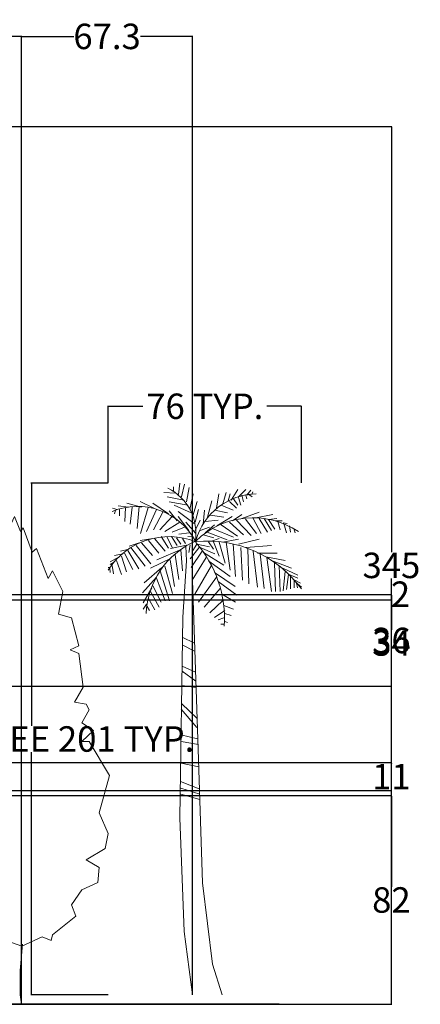
# Model space of a CAD drawing. Units: inches. Extents: x 403 to 1256, y 451 to 842.
# Tile 4 of 4: x 1098 to 1256, y 455 to 842. Entities that reach past the tile are written whole.
import ezdxf

# ---------------------------------------------------------------- set-up
doc = ezdxf.new("R2010")
doc.units = ezdxf.units.IN
doc.header["$MEASUREMENT"] = 0
for name, color, linetype, lineweight in [('A-ANNO-DIMS', 2, 'Continuous', 18), ('A-WALL', 7, 'Continuous', 35), ('PLANTS', 3, 'Continuous', 18)]:
    doc.layers.add(name, color=color, linetype=linetype, lineweight=lineweight)
doc.styles.get("Standard").update_dxf_attribs({"font": 'arial.ttf'})
doc.dimstyles.get("Standard").update_dxf_attribs({"dimtxt": 10, "dimasz": 0.18, "dimexe": 0.18, "dimexo": 0.0625, "dimgap": 0.09, "dimtad": 0, "dimtih": 1, "dimtoh": 1, "dimdec": 0, "dimzin": 0, "dimdsep": 46, "dimlunit": 3, "dimtxsty": 'Standard', "dimcen": 0.09, "dimadec": 0, "dimazin": 0, "dimtfac": 1, "dimtdec": 0, "dimtofl": 0, "dimtmove": 0, "dimatfit": 3, "dimfxl": 1, "dimtolj": 1, "dimtzin": 0, "dimarcsym": 0})

# ---------------------------------------------------------------- blocks, each defined once
blk = doc.blocks.new('Tree - palm elevation')
for p, q in [((-6.727, 197.202), (-11.366, 197.45)), ((-7.5, 199.68), (-7.5, 197.946)), ((-5.567, 196.707), (-4.987, 201.167)), ((-4.407, 195.716), (-3.247, 200.672)), ((-2.474, 193.733), (-1.315, 199.433)), ((11.829, 192.99), (13.182, 197.45)), ((15.116, 194.477), (17.822, 198.689)), ((18.015, 195.716), (20.914, 198.689)), ((21.301, 196.459), (22.847, 198.441)), ((23.234, 196.707), (23.62, 197.698)), ((-15.232, 191.255), (-20.644, 193.981)), ((-3.441, 194.477), (-10.013, 195.716)), ((-1.894, 192.494), (-9.24, 193.733)), ((-1.121, 190.759), (0.232, 196.955)), ((0.038, 188.281), (1.778, 193.981)), ((5.837, 187.786), (7.577, 194.229)), ((9.317, 191.255), (10.283, 196.955)), ((13.956, 194.229), (14.729, 196.955)), ((14.536, 193.981), (17.242, 191.255)), ((16.082, 194.972), (17.822, 192.494)), ((18.015, 195.468), (18.981, 192.494)), ((19.368, 196.459), (19.948, 193.733)), ((20.914, 196.459), (21.301, 194.972)), ((22.074, 196.707), (23.427, 195.716)), ((-29.729, 190.759), (-31.469, 191.255)), ((-30.309, 190.512), (-30.695, 189.025)), ((-25.283, 191.751), (-29.342, 192.246)), ((-28.763, 190.759), (-28.763, 188.281)), ((-26.443, 191.503), (-26.636, 186.051)), ((-20.064, 191.751), (-25.863, 193.238)), ((-23.737, 191.751), (-24.51, 185.06)), ((-21.031, 191.998), (-21.804, 183.325)), ((-17.551, 191.503), (-20.451, 181.343)), ((-14.265, 190.759), (-18.131, 182.086)), ((-9.433, 189.025), (-15.618, 193.238)), ((-11.753, 189.768), (-15.425, 182.83)), ((-6.147, 186.299), (-9.24, 190.264)), ((-0.541, 189.52), (-7.307, 192.494)), ((-5.76, 190.016), (0.618, 185.308)), ((1.005, 185.803), (2.358, 190.759)), ((4.098, 185.06), (4.678, 190.512)), ((8.544, 190.512), (13.763, 189.52)), ((11.25, 192.494), (15.889, 190.512)), ((19.368, 187.29), (26.133, 189.768)), ((-8.08, 188.034), (-12.912, 182.83)), ((-4.987, 185.803), (-10.979, 182.086)), ((-5.76, 188.034), (-1.508, 182.582)), ((-2.668, 185.803), (1.198, 181.343)), ((1.005, 182.582), (2.938, 186.547)), ((4.871, 186.051), (10.09, 186.547)), ((6.997, 188.529), (12.216, 187.786)), ((9.51, 184.317), (15.502, 188.034)), ((14.536, 185.803), (19.948, 180.847)), ((15.695, 186.299), (19.368, 188.777)), ((17.242, 186.547), (23.041, 180.599)), ((20.721, 187.042), (25.167, 181.343)), ((23.814, 187.29), (26.907, 181.343)), ((24.78, 187.538), (31.546, 188.777)), ((26.133, 187.29), (29.419, 181.838)), ((28.066, 187.29), (30.966, 182.582)), ((29.806, 186.795), (32.319, 183.078)), ((29.999, 186.795), (33.092, 187.29)), ((32.512, 186.299), (35.218, 186.299)), ((33.479, 186.051), (34.445, 182.83)), ((-3.247, 183.821), (-8.08, 181.838)), ((2.938, 182.582), (6.61, 183.821)), ((4.871, 181.591), (8.544, 184.812)), ((7.77, 183.325), (16.082, 179.856)), ((11.25, 184.812), (17.628, 180.352)), ((35.605, 185.556), (37.151, 185.308)), ((35.798, 185.308), (36.958, 181.591)), ((38.118, 184.317), (38.504, 181.838)), ((39.857, 182.83), (40.244, 181.591)), ((-15.618, 179.36), (-20.644, 178.617)), ((-17.358, 178.617), (-13.299, 173.661)), ((-15.038, 179.36), (-10.786, 174.404)), ((-12.332, 180.104), (-9.433, 175.643)), ((-10.206, 180.104), (-8.08, 175.891)), ((-8.273, 180.104), (-6.147, 176.635)), ((-6.34, 179.608), (-4.6, 177.13)), ((-1.315, 181.591), (-5.374, 181.095)), ((-4.021, 179.36), (-2.861, 177.378)), ((-0.348, 180.352), (-1.894, 180.104)), ((4.098, 180.847), (8.35, 179.608)), ((5.644, 181.838), (13.569, 178.865)), ((6.224, 178.121), (8.157, 175.148)), ((7.384, 178.369), (10.476, 179.36)), ((8.157, 178.121), (10.476, 172.422)), ((11.829, 177.874), (18.015, 179.113)), ((18.015, 177.13), (26.133, 179.113)), ((-25.09, 175.148), (-28.376, 174.404)), ((-25.476, 174.652), (-21.224, 167.466)), ((-21.031, 177.626), (-24.897, 176.387)), ((-24.317, 175.891), (-18.711, 168.457)), ((-22.191, 176.635), (-16.391, 169.448)), ((-20.064, 177.626), (-15.812, 172.67)), ((-4.214, 175.148), (-14.072, 170.935)), ((-1.701, 176.882), (-8.66, 175.396)), ((-4.6, 174.9), (-4.021, 166.722)), ((-2.668, 176.387), (-2.376, 170.594)), ((-0.928, 176.882), (-1.508, 173.909)), ((2.551, 175.891), (-0.928, 171.431)), ((3.711, 174.404), (-0.541, 167.961)), ((1.585, 177.13), (0.038, 174.652)), ((1.585, 177.13), (6.61, 176.139)), ((2.938, 175.891), (8.737, 173.413)), ((10.476, 177.874), (12.796, 169.696)), ((13.182, 177.874), (14.729, 166.97)), ((15.889, 177.13), (16.855, 164.492)), ((18.981, 175.891), (19.561, 163.005)), ((20.914, 175.891), (30.966, 176.635)), ((21.688, 175.396), (22.074, 161.518)), ((23.814, 174.404), (25.554, 160.279)), ((-28.956, 172.174), (-32.435, 170.192)), ((-27.409, 173.413), (-30.695, 172.67)), ((-29.922, 170.687), (-27.989, 165.235)), ((-27.989, 172.422), (-26.056, 166.227)), ((-26.829, 173.661), (-23.544, 167.218)), ((-8.466, 171.678), (-16.585, 167.713)), ((-8.853, 170.935), (-7.113, 160.527)), ((-6.92, 172.917), (-5.374, 163.253)), ((5.257, 171.926), (-0.155, 163.005)), ((4.291, 173.909), (12.216, 168.953)), ((6.417, 170.439), (14.729, 164.492)), ((25.554, 173.661), (33.285, 173.661)), ((26.52, 173.165), (28.066, 159.784)), ((28.839, 172.174), (36.378, 170.687)), ((29.226, 171.926), (30.966, 158.545)), ((30.966, 170.687), (38.891, 167.713)), ((-32.628, 167.961), (-33.208, 167.961)), ((-32.628, 167.713), (-32.435, 165.979)), ((-31.082, 169.944), (-32.435, 169.2)), ((-31.662, 168.705), (-31.082, 165.483)), ((-12.139, 167.961), (-19.098, 162.014)), ((-12.719, 166.722), (-9.046, 154.828)), ((-10.979, 168.457), (-7.887, 157.801)), ((7.384, 168.705), (0.812, 157.553)), ((32.126, 169.696), (32.512, 158.545)), ((34.058, 168.705), (34.445, 158.545)), ((35.412, 167.713), (41.404, 164.988)), ((36.378, 166.474), (35.605, 158.792)), ((-14.265, 164.244), (-19.678, 158.049)), ((-14.265, 163.749), (-10.786, 154.828)), ((9.317, 164.244), (2.358, 154.332)), ((8.544, 165.979), (16.662, 160.527)), ((37.731, 165.235), (36.958, 159.288)), ((37.924, 165.235), (41.404, 163.749)), ((38.504, 164.492), (38.504, 159.536)), ((39.664, 163.253), (42.37, 161.766)), ((39.857, 162.757), (39.857, 160.031)), ((-16.005, 160.031), (-19.484, 154.084)), ((-15.618, 160.775), (-12.332, 154.332)), ((10.863, 159.784), (4.484, 152.35)), ((10.09, 162.51), (17.435, 157.058)), ((40.824, 161.766), (41.21, 160.031)), ((41.21, 161.518), (42.757, 160.279)), ((-17.358, 155.819), (-14.845, 151.358)), ((-16.585, 158.545), (-13.106, 152.35)), ((11.829, 155.075), (6.804, 150.119)), ((11.443, 157.553), (16.855, 154.332)), ((-18.131, 153.589), (-19.484, 151.606)), ((-17.938, 152.597), (-16.972, 151.111)), ((12.603, 151.111), (8.544, 148.385)), ((12.216, 153.093), (16.082, 151.606)), ((12.216, 148.137), (10.09, 147.393)), ((12.603, 149.872), (15.116, 149.128)), ((12.409, 145.659), (11.056, 145.659)), ((12.409, 146.898), (13.763, 146.402)), ((-4.081, 140.645), (0.753, 138.261)), ((-4.081, 137.547), (0.753, 135.163)), ((-4.081, 129.205), (1.124, 126.821)), ((-4.081, 127.298), (1.31, 123.246)), ((-4.081, 121.578), (1.31, 120.863)), ((-4.453, 112.283), (1.682, 105.133)), ((-4.267, 114.428), (1.682, 108.708)), ((-4.639, 102.273), (1.868, 100.604)), ((-4.453, 99.651), (2.24, 98.459)), ((-4.453, 91.071), (2.426, 89.641)), ((-4.825, 83.921), (2.612, 81.061)), ((-4.639, 81.299), (2.797, 78.916)), ((-4.639, 78.916), (2.797, 76.771))]:
    blk.add_line(p, q)
for points in [[(-2.363, 170.553), (-3.88, 148.505), (-4.988, 69.634), (-3.325, 24.869), (0, 0)], [(-0.116, 162.848), (0.554, 143.532), (2.217, 96.635), (3.88, 44.054), (7.76, 12.079), (11.64, 0)]]:
    blk.add_lwpolyline(points)
for centre, radius, start, end in [((-18.427, 181.448), 19.715, 350.285, 64.11229), ((25.595, 171.567), 25.395, 91.40319, 163.882), ((-21.738, 166.094), 25.899, 27.67115, 112.5305), ((23.687, 155.341), 32.188, 56.19272, 134.3213), ((-9.259, 151.732), 28.386, 68.38311, 147.5322), ((14.394, 148.393), 32.752, 113.7592, 177.4133), ((5.828, 132.718), 45.639, 35.98777, 95.82273), ((-32.8, 147.923), 45.309, 356.1943, 41.37848)]:
    blk.add_arc(centre, radius, start, end)
blk = doc.blocks.new('Tree - type 2 deciduous elevation')
blk.add_lwpolyline([(-2.754, 191.699), (-6.78, 182.851), (-13.682, 176.953), (-11.956, 173.266), (-9.656, 172.529), (-14.257, 170.317), (-13.682, 167.368), (-21.733, 157.783), (-25.184, 154.834), (-21.158, 150.41), (-21.733, 147.461), (-22.884, 140.825), (-26.334, 140.087), (-29.21, 134.926), (-28.635, 129.028), (-32.661, 128.291), (-36.111, 120.18), (-34.386, 118.706), (-35.536, 111.333), (-38.987, 106.171), (-34.386, 107.646), (-40.712, 98.798), (-37.261, 95.849), (-40.712, 90.688), (-41.287, 80.366), (-38.412, 78.154), (-36.686, 70.781), (-39.562, 71.518), (-37.261, 64.145), (-38.412, 57.509), (-36.111, 58.247), (-33.236, 52.348), (-35.536, 53.086), (-34.961, 46.45), (-30.36, 44.975), (-31.51, 36.128), (-26.334, 36.865), (-23.459, 39.814), (-18.283, 36.128), (-20.008, 33.178), (-14.832, 31.704), (-11.956, 33.178), (-12.531, 27.28), (-6.205, 22.856), (-3.905, 24.331), (0.121, 22.856), (8.173, 26.543), (11.624, 25.068), (12.199, 27.28), (21.4, 34.653), (19.675, 39.077), (23.701, 44.975), (30.027, 47.924), (30.602, 53.823), (25.426, 56.772), (32.903, 61.196), (34.053, 67.094), (30.602, 75.205), (34.628, 89.951), (26.576, 103.222), (23.701, 103.222), (28.302, 107.646), (23.701, 110.595), (26.576, 115.756), (25.426, 117.968), (20.825, 118.706), (24.276, 124.604), (22.551, 137.876), (19.1, 139.35), (22.551, 140.825), (19.675, 151.884), (14.499, 153.359), (16.224, 162.207), (12.199, 170.317), (10.473, 167.368), (5.872, 179.165), (4.147, 177.69), (0.696, 187.275), (-0.454, 185.8)], close=True)
for points in [[(-6.813, 23.669), (-6.813, 11.669), (-8.627, 0)], [(0.387, 23.669), (-0.576, 13.271), (-0.576, 3.686), (0, 0)]]:
    blk.add_lwpolyline(points)
blk = doc.blocks.new('*D7')
at = {"layer": 'A-ANNO-DIMS', "color": 0, "lineweight": -2, "transparency": 16777216}
for p, q in [((1132.84, 659.81), (1102.54, 659.81)), ((1102.72, 659.63), (1102.72, 564.43)), ((1102.72, 458.83), (1102.72, 554.04)), ((1132.84, 458.65), (1102.54, 458.65))]:
    blk.add_line(p, q, dxfattribs=at)
at = {"layer": 'A-ANNO-DIMS', "color": 0, "transparency": 16777216}
for points in [[(1102.69, 659.63), (1102.75, 659.63), (1102.72, 659.81)], [(1102.69, 458.83), (1102.75, 458.83), (1102.72, 458.65)]]:
    blk.add_solid(points, dxfattribs=at)
at = {"layer": 'Defpoints', "color": 0, "transparency": 16777216}
for p in [(1102.72, 659.81), (1132.9, 659.81), (1132.9, 458.65)]:
    blk.add_point(p, dxfattribs=at)
at = {"layer": 'A-ANNO-DIMS', "color": 0, "transparency": 16777216, "insert": (1102.72, 559.23), "char_height": 10, "attachment_point": 5}
blk.add_mtext('\\A1;PALM TREE 201 TYP.', dxfattribs=at)
blk = doc.blocks.new('*D8')
at = {"layer": 'A-ANNO-DIMS', "color": 0, "lineweight": -2, "transparency": 16777216}
for p, q in [((1132.9, 659.88), (1132.9, 690.17)), ((1133.08, 689.99), (1146.49, 689.99)), ((1208.68, 689.99), (1195.27, 689.99)), ((1208.86, 659.88), (1208.86, 690.17))]:
    blk.add_line(p, q, dxfattribs=at)
at = {"layer": 'A-ANNO-DIMS', "color": 0, "transparency": 16777216}
for points in [[(1133.08, 690.02), (1133.08, 689.96), (1132.9, 689.99)], [(1208.68, 690.02), (1208.68, 689.96), (1208.86, 689.99)]]:
    blk.add_solid(points, dxfattribs=at)
at = {"layer": 'Defpoints', "color": 0, "transparency": 16777216}
for p in [(1208.86, 689.99), (1132.9, 659.81), (1208.86, 659.81)]:
    blk.add_point(p, dxfattribs=at)
at = {"layer": 'A-ANNO-DIMS', "color": 0, "transparency": 16777216, "insert": (1170.88, 689.99), "char_height": 10, "attachment_point": 5}
blk.add_mtext('\\A1;76 TYP.', dxfattribs=at)
blk = doc.blocks.new('*D12')
at = {"layer": 'A-ANNO-DIMS', "color": 0, "lineweight": -2, "transparency": 16777216}
for p, q in [((966.02, 799.96), (1244.44, 799.96)), ((1244.26, 799.78), (1244.26, 632.66)), ((1244.26, 455.14), (1244.26, 622.26)), ((1042.52, 454.96), (1244.44, 454.96))]:
    blk.add_line(p, q, dxfattribs=at)
at = {"layer": 'A-ANNO-DIMS', "color": 0, "transparency": 16777216}
for points in [[(1244.23, 799.78), (1244.29, 799.78), (1244.26, 799.96)], [(1244.23, 455.14), (1244.29, 455.14), (1244.26, 454.96)]]:
    blk.add_solid(points, dxfattribs=at)
at = {"layer": 'Defpoints', "color": 0, "transparency": 16777216}
for p in [(965.96, 799.96), (1244.26, 799.96), (1042.46, 454.96)]:
    blk.add_point(p, dxfattribs=at)
at = {"layer": 'A-ANNO-DIMS', "color": 0, "transparency": 16777216, "insert": (1244.26, 627.46), "char_height": 10, "attachment_point": 5}
blk.add_mtext('\\A1;345', dxfattribs=at)
blk = doc.blocks.new('*D20')
at = {"layer": 'A-ANNO-DIMS', "color": 0, "lineweight": -2, "transparency": 16777216}
for p, q in [((706.52, 615.96), (1244.44, 615.96)), ((1244.26, 615.78), (1244.26, 603.16)), ((1244.26, 580.14), (1244.26, 592.76)), ((682.52, 579.96), (1244.44, 579.96))]:
    blk.add_line(p, q, dxfattribs=at)
at = {"layer": 'A-ANNO-DIMS', "color": 0, "transparency": 16777216}
for points in [[(1244.23, 615.78), (1244.29, 615.78), (1244.26, 615.96)], [(1244.23, 580.14), (1244.29, 580.14), (1244.26, 579.96)]]:
    blk.add_solid(points, dxfattribs=at)
at = {"layer": 'Defpoints', "color": 0, "transparency": 16777216}
for p in [(706.46, 615.96), (1244.26, 615.96), (682.46, 579.96)]:
    blk.add_point(p, dxfattribs=at)
at = {"layer": 'A-ANNO-DIMS', "color": 0, "transparency": 16777216, "insert": (1244.26, 597.96), "char_height": 10, "attachment_point": 5}
blk.add_mtext('\\A1;36', dxfattribs=at)
blk = doc.blocks.new('*D30')
at = {"layer": 'A-ANNO-DIMS', "color": 0, "lineweight": -2, "transparency": 16777216}
for p, q in [((1042.46, 455.02), (1042.46, 835.54)), ((1042.64, 835.36), (1053.63, 835.36)), ((1098.63, 835.36), (1087.63, 835.36)), ((1098.81, 455.02), (1098.81, 835.54))]:
    blk.add_line(p, q, dxfattribs=at)
at = {"layer": 'A-ANNO-DIMS', "color": 0, "transparency": 16777216}
for points in [[(1042.64, 835.39), (1042.64, 835.33), (1042.46, 835.36)], [(1098.63, 835.39), (1098.63, 835.33), (1098.81, 835.36)]]:
    blk.add_solid(points, dxfattribs=at)
at = {"layer": 'Defpoints', "color": 0, "transparency": 16777216}
for p in [(1098.81, 835.36), (1042.46, 454.96), (1098.81, 454.96)]:
    blk.add_point(p, dxfattribs=at)
at = {"layer": 'A-ANNO-DIMS', "color": 0, "transparency": 16777216, "insert": (1070.63, 835.36), "char_height": 10, "attachment_point": 5}
blk.add_mtext('\\A1;56.35', dxfattribs=at)
blk = doc.blocks.new('*D31')
at = {"layer": 'A-ANNO-DIMS', "color": 0, "lineweight": -2, "transparency": 16777216}
for p, q in [((1098.81, 455.02), (1098.81, 835.54)), ((1098.99, 835.36), (1119.35, 835.36)), ((1165.93, 835.36), (1145.56, 835.36)), ((1166.11, 458.71), (1166.11, 835.54))]:
    blk.add_line(p, q, dxfattribs=at)
at = {"layer": 'A-ANNO-DIMS', "color": 0, "transparency": 16777216}
for points in [[(1098.99, 835.39), (1098.99, 835.33), (1098.81, 835.36)], [(1165.93, 835.39), (1165.93, 835.33), (1166.11, 835.36)]]:
    blk.add_solid(points, dxfattribs=at)
at = {"layer": 'Defpoints', "color": 0, "transparency": 16777216}
for p in [(1166.11, 835.36), (1166.11, 458.65), (1098.81, 454.96)]:
    blk.add_point(p, dxfattribs=at)
at = {"layer": 'A-ANNO-DIMS', "color": 0, "transparency": 16777216, "insert": (1132.46, 835.36), "char_height": 10, "attachment_point": 5}
blk.add_mtext('\\A1;67.3', dxfattribs=at)
blk = doc.blocks.new('*D32')
at = {"layer": 'A-ANNO-DIMS', "color": 0, "lineweight": -2, "transparency": 16777216}
for p, q in [((1031.52, 536.96), (1244.44, 536.96)), ((1244.26, 536.78), (1244.26, 501.16)), ((1244.26, 455.14), (1244.26, 490.77)), ((1031.52, 454.96), (1244.44, 454.96))]:
    blk.add_line(p, q, dxfattribs=at)
at = {"layer": 'A-ANNO-DIMS', "color": 0, "transparency": 16777216}
for points in [[(1244.23, 536.78), (1244.29, 536.78), (1244.26, 536.96)], [(1244.23, 455.14), (1244.29, 455.14), (1244.26, 454.96)]]:
    blk.add_solid(points, dxfattribs=at)
at = {"layer": 'Defpoints', "color": 0, "transparency": 16777216}
for p in [(1031.46, 536.96), (1244.26, 536.96), (1031.46, 454.96)]:
    blk.add_point(p, dxfattribs=at)
at = {"layer": 'A-ANNO-DIMS', "color": 0, "transparency": 16777216, "insert": (1244.26, 495.96), "char_height": 10, "attachment_point": 5}
blk.add_mtext('\\A1;82', dxfattribs=at)
blk = doc.blocks.new('*D34')
at = {"layer": 'A-ANNO-DIMS', "color": 0, "lineweight": -2, "transparency": 16777216}
for p, q in [((885.02, 549.96), (1244.44, 549.96)), ((1244.26, 549.78), (1244.26, 549.57)), ((886.02, 538.96), (1244.44, 538.96)), ((1244.26, 539.14), (1244.26, 539.35))]:
    blk.add_line(p, q, dxfattribs=at)
at = {"layer": 'A-ANNO-DIMS', "color": 0, "transparency": 16777216}
for points in [[(1244.23, 549.78), (1244.29, 549.78), (1244.26, 549.96)], [(1244.23, 539.14), (1244.29, 539.14), (1244.26, 538.96)]]:
    blk.add_solid(points, dxfattribs=at)
at = {"layer": 'Defpoints', "color": 0, "transparency": 16777216}
for p in [(884.96, 549.96), (1244.26, 549.96), (885.96, 538.96)]:
    blk.add_point(p, dxfattribs=at)
at = {"layer": 'A-ANNO-DIMS', "color": 0, "transparency": 16777216, "insert": (1244.26, 544.46), "char_height": 10, "attachment_point": 5}
blk.add_mtext('\\A1;11', dxfattribs=at)
blk = doc.blocks.new('*D40')
at = {"layer": 'A-ANNO-DIMS', "color": 0, "lineweight": -2, "transparency": 16777216}
for p, q in [((894.52, 613.96), (1244.44, 613.96)), ((1244.26, 613.78), (1244.26, 602.16)), ((1244.26, 580.14), (1244.26, 591.76)), ((894.52, 579.96), (1244.44, 579.96))]:
    blk.add_line(p, q, dxfattribs=at)
at = {"layer": 'A-ANNO-DIMS', "color": 0, "transparency": 16777216}
for points in [[(1244.23, 613.78), (1244.29, 613.78), (1244.26, 613.96)], [(1244.23, 580.14), (1244.29, 580.14), (1244.26, 579.96)]]:
    blk.add_solid(points, dxfattribs=at)
at = {"layer": 'Defpoints', "color": 0, "transparency": 16777216}
for p in [(894.46, 613.96), (1244.26, 613.96), (894.46, 579.96)]:
    blk.add_point(p, dxfattribs=at)
at = {"layer": 'A-ANNO-DIMS', "color": 0, "transparency": 16777216, "insert": (1244.26, 596.96), "char_height": 10, "attachment_point": 5}
blk.add_mtext('\\A1;34', dxfattribs=at)
blk = doc.blocks.new('*D41')
at = {"layer": 'A-ANNO-DIMS', "color": 0, "lineweight": -2, "transparency": 16777216}
for p, q in [((894.52, 615.96), (1244.44, 615.96)), ((1244.26, 615.96), (1244.26, 616.14)), ((1244.26, 616.14), (1244.44, 616.14)), ((1244.26, 614.14), (1244.26, 615.78)), ((894.52, 613.96), (1244.44, 613.96))]:
    blk.add_line(p, q, dxfattribs=at)
at = {"layer": 'A-ANNO-DIMS', "color": 0, "transparency": 16777216}
for points in [[(1244.23, 615.78), (1244.29, 615.78), (1244.26, 615.96)], [(1244.23, 614.14), (1244.29, 614.14), (1244.26, 613.96)]]:
    blk.add_solid(points, dxfattribs=at)
at = {"layer": 'Defpoints', "color": 0, "transparency": 16777216}
for p in [(894.46, 615.96), (1244.26, 615.96), (894.46, 613.96)]:
    blk.add_point(p, dxfattribs=at)
at = {"layer": 'A-ANNO-DIMS', "color": 0, "transparency": 16777216, "insert": (1247.85, 616.14), "char_height": 10, "attachment_point": 5}
blk.add_mtext('\\A1;2', dxfattribs=at)

msp = doc.modelspace()

# ---------------------------------------------------------------- linework, layer by layer
at = {"layer": 'A-WALL'}
msp.add_line((1042.459, 454.9615), (1200.0763, 454.9615), dxfattribs=at)

# ---------------------------------------------------------------- block references
at = {"layer": 'PLANTS'}
for name, p in [('Tree - palm elevation', (1166.107, 458.6475)), ('Tree - type 2 deciduous elevation', (1098.8106, 454.9615))]:
    msp.add_blockref(name, p, dxfattribs=at)

# ---------------------------------------------------------------- dimensions: what is measured, and where the dimension line sits
at = {"layer": 'A-ANNO-DIMS'}
for base, p1, p2, override, picture, middle in [((1098.8106, 835.3615), (1042.459, 454.9615), (1098.8106, 454.9615), {"dimdec": 2, "dimlfac": 1, "dimrnd": 0, "dimzin": 0, "dimdsep": 46, "dimlunit": 2}, '*D30', (1070.6348, 835.3615)), ((1166.107, 835.3615), (1098.8106, 454.9615), (1166.107, 458.6475), {"dimdec": 1, "dimlfac": 1, "dimrnd": 0, "dimzin": 0, "dimdsep": 46, "dimlunit": 2}, '*D31', (1132.4588, 835.3615))]:
    dim = msp.add_linear_dim(base=base, p1=p1, p2=p2, dimstyle='Standard', override=override, dxfattribs=at)
    dim.commit()
    dim.dimension.update_dxf_attribs({"geometry": picture, "text_midpoint": middle})
for base, p1, p2, picture, middle in [((1244.264, 799.9615), (1042.459, 454.9615), (965.959, 799.9615), '*D12', (1244.264, 627.4615)), ((1244.264, 615.9615), (894.459, 613.9615), (894.459, 615.9615), '*D41', (1247.8458, 616.1415)), ((1244.264, 615.9615), (682.459, 579.9615), (706.459, 615.9615), '*D20', (1244.264, 597.9615)), ((1244.264, 613.9615), (894.459, 579.9615), (894.459, 613.9615), '*D40', (1244.264, 596.9615)), ((1244.264, 549.9615), (885.959, 538.9615), (884.959, 549.9615), '*D34', (1244.264, 544.4615)), ((1244.264, 536.9615), (1031.459, 454.9615), (1031.459, 536.9615), '*D32', (1244.264, 495.9615))]:
    dim = msp.add_linear_dim(base=base, p1=p1, p2=p2, angle=90, dimstyle='Standard', override={"dimdec": 0, "dimlfac": 1, "dimrnd": 0, "dimzin": 0, "dimdsep": 46, "dimlunit": 2}, dxfattribs=at)
    dim.commit()
    dim.dimension.update_dxf_attribs({"geometry": picture, "text_midpoint": middle})
dim = msp.add_linear_dim(base=(1208.864, 689.9896), p1=(1132.8989, 659.8145), p2=(1208.864, 659.8145), text='<> TYP.', dimstyle='Standard', override={"dimdec": 0, "dimlfac": 1, "dimrnd": 0, "dimzin": 0, "dimdsep": 46, "dimlunit": 2}, dxfattribs=at)
dim.commit()
dim.dimension.update_dxf_attribs({"geometry": '*D8', "text_midpoint": (1170.8815, 689.9896)})
dim = msp.add_linear_dim(base=(1102.7239, 659.8145), p1=(1132.8989, 458.6475), p2=(1132.8989, 659.8145), angle=90, text='PALM TREE <> TYP.', dimstyle='Standard', override={"dimdec": 0, "dimlfac": 1, "dimrnd": 0, "dimzin": 0, "dimdsep": 46, "dimlunit": 2}, dxfattribs=at)
dim.commit()
dim.dimension.update_dxf_attribs({"geometry": '*D7', "text_midpoint": (1102.7239, 559.231)})

doc.saveas('drawing.dxf')
